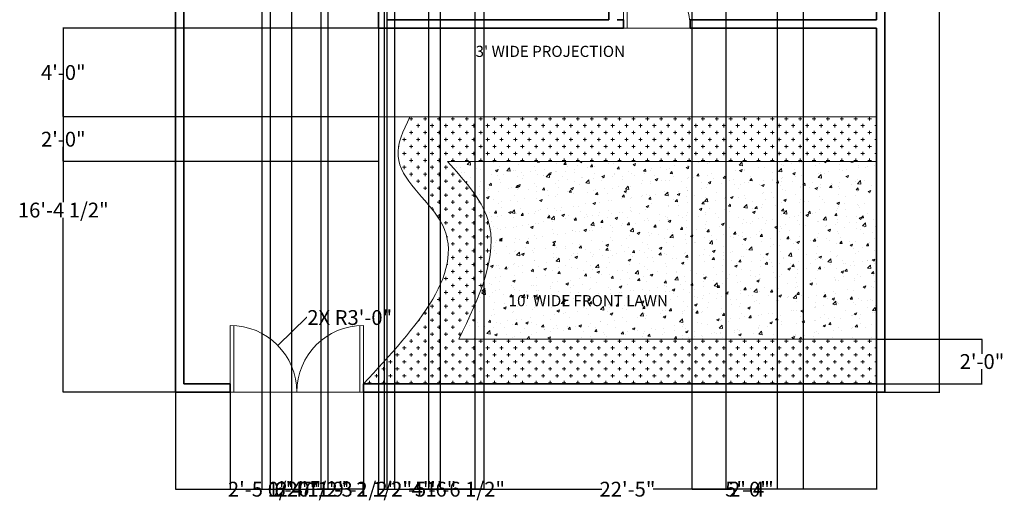
# Model space of a CAD drawing. Units: inches. Extents: x -438 to 102, y -60 to 1091.
# Tile 1 of 20: x -438 to 93, y -60 to 205. Entities that reach past the tile are written whole.
import ezdxf

# ---------------------------------------------------------------- set-up
doc = ezdxf.new("R2010")
doc.units = ezdxf.units.IN
doc.header["$MEASUREMENT"] = 0
for name, color, linetype, lineweight, true_color in [('A-ANNO-DIMS', 217, 'Continuous', 18, 0x93278f), ('A-DOOR', 30, 'Continuous', 18, 0xf26722), ('A-WALL', 2, 'Continuous', 35, 0xf1eb1f), ('C-PROP', 2, 'Continuous', 35, 0xf1eb1f), ('L-PLNT-PATT', 85, 'Continuous', 13, 0x58ba48)]:
    doc.layers.add(name, color=color, linetype=linetype, lineweight=lineweight, true_color=true_color)
for name, color, linetype, lineweight in [('A-AREA-IDEN', 4, 'Continuous', 18), ('C-SITE-GATE', 7, 'Continuous', 18), ('C-SITE-PVMT', 7, 'Continuous', 18), ('L-PLNT', 85, 'Continuous', 18)]:
    doc.layers.add(name, color=color, linetype=linetype, lineweight=lineweight)
doc.styles.get("Standard").update_dxf_attribs({"font": 'arial.ttf'})
doc.dimstyles.get("Standard").update_dxf_attribs({"dimtxt": 8, "dimasz": 0.18, "dimexe": 0.18, "dimexo": 0.0625, "dimgap": 0.09, "dimtad": 0, "dimtih": 1, "dimtoh": 1, "dimdec": 4, "dimzin": 0, "dimdsep": 46, "dimlunit": 3, "dimtxsty": 'Standard', "dimcen": 0.09, "dimadec": 0, "dimazin": 0, "dimtfac": 1, "dimtdec": 4, "dimtofl": 0, "dimtmove": 0, "dimatfit": 3, "dimfxl": 1, "dimtolj": 1, "dimtzin": 0, "dimarcsym": 0})

# ---------------------------------------------------------------- blocks, each defined once
blk = doc.blocks.new('*D5')
at = {"layer": 'A-ANNO-DIMS', "color": 0, "lineweight": -2, "transparency": 16777216}
for p, q in [((28.92, 1027), (58.42, 1027)), ((58.24, 1026.82), (58.24, 519.68)), ((58.24, 4.18), (58.24, 511.32)), ((28.92, 4), (58.42, 4))]:
    blk.add_line(p, q, dxfattribs=at)
at = {"layer": 'A-ANNO-DIMS', "color": 0, "transparency": 16777216}
for points in [[(58.21, 1026.82), (58.27, 1026.82), (58.24, 1027)], [(58.21, 4.18), (58.27, 4.18), (58.24, 4)]]:
    blk.add_solid(points, dxfattribs=at)
at = {"layer": 'Defpoints', "color": 0, "transparency": 16777216}
for p in [(28.85, 1027), (28.85, 4), (58.24, 4)]:
    blk.add_point(p, dxfattribs=at)
at = {"layer": 'A-ANNO-DIMS', "color": 0, "transparency": 16777216, "insert": (58.24, 515.5), "char_height": 8, "attachment_point": 5}
blk.add_mtext('\\A1;85\'-3.0000"', dxfattribs=at)
blk = doc.blocks.new('DOOR-SWING-36')
for p, q in [((-36, 0), (0, 0)), ((-2, 0), (-2, -36)), ((0, 0), (0, -36))]:
    blk.add_line(p, q)
blk.add_arc((0, 0), 36, 180, 270)
blk = doc.blocks.new('*D24')
at = {"layer": 'A-ANNO-DIMS', "color": 0, "lineweight": -2, "transparency": 16777216}
for p, q in [((-354.15, 3.94), (-354.15, -48.58)), ((-324.71, 3.94), (-324.71, -48.58)), ((-353.97, -48.4), (-324.89, -48.4)), ((-324.71, -48.4), (-324.53, -48.4))]:
    blk.add_line(p, q, dxfattribs=at)
at = {"layer": 'A-ANNO-DIMS', "color": 0, "transparency": 16777216}
for points in [[(-353.97, -48.37), (-353.97, -48.43), (-354.15, -48.4)], [(-324.89, -48.37), (-324.89, -48.43), (-324.71, -48.4)]]:
    blk.add_solid(points, dxfattribs=at)
at = {"layer": 'Defpoints', "color": 0, "transparency": 16777216}
for p in [(-354.15, 4), (-324.71, 4), (-324.71, -48.4)]:
    blk.add_point(p, dxfattribs=at)
at = {"layer": 'A-ANNO-DIMS', "color": 0, "transparency": 16777216, "insert": (-304.42, -48.4), "char_height": 8, "attachment_point": 5}
blk.add_mtext('\\A1;2\'-5 1/2"', dxfattribs=at)
blk = doc.blocks.new('*D25')
at = {"layer": 'A-ANNO-DIMS', "color": 0, "lineweight": -2, "transparency": 16777216}
for p, q in [((-324.71, 3.94), (-324.71, -48.58)), ((-252.71, 3.94), (-252.71, -48.58)), ((-324.53, -48.4), (-299.45, -48.4)), ((-252.89, -48.4), (-277.96, -48.4))]:
    blk.add_line(p, q, dxfattribs=at)
at = {"layer": 'A-ANNO-DIMS', "color": 0, "transparency": 16777216}
for points in [[(-324.53, -48.37), (-324.53, -48.43), (-324.71, -48.4)], [(-252.89, -48.37), (-252.89, -48.43), (-252.71, -48.4)]]:
    blk.add_solid(points, dxfattribs=at)
at = {"layer": 'Defpoints', "color": 0, "transparency": 16777216}
for p in [(-324.71, 4), (-252.71, 4), (-252.71, -48.4)]:
    blk.add_point(p, dxfattribs=at)
at = {"layer": 'A-ANNO-DIMS', "color": 0, "transparency": 16777216, "insert": (-288.71, -48.4), "char_height": 8, "attachment_point": 5}
blk.add_mtext('\\A1;6\'-0"', dxfattribs=at)
blk = doc.blocks.new('*D26')
at = {"layer": 'A-ANNO-DIMS', "color": 0, "lineweight": -2, "transparency": 16777216}
for p, q in [((-244.65, 200.44), (-244.65, -48.58)), ((24.35, 200.44), (24.35, -48.58)), ((-244.47, -48.4), (-124.05, -48.4)), ((24.17, -48.4), (-96.25, -48.4))]:
    blk.add_line(p, q, dxfattribs=at)
at = {"layer": 'A-ANNO-DIMS', "color": 0, "transparency": 16777216}
for points in [[(-244.47, -48.37), (-244.47, -48.43), (-244.65, -48.4)], [(24.17, -48.37), (24.17, -48.43), (24.35, -48.4)]]:
    blk.add_solid(points, dxfattribs=at)
at = {"layer": 'Defpoints', "color": 0, "transparency": 16777216}
for p in [(-244.65, 200.5), (24.35, 200.5), (24.35, -48.4)]:
    blk.add_point(p, dxfattribs=at)
at = {"layer": 'A-ANNO-DIMS', "color": 0, "transparency": 16777216, "insert": (-110.15, -48.4), "char_height": 8, "attachment_point": 5}
blk.add_mtext('\\A1;22\'-5"', dxfattribs=at)
blk = doc.blocks.new('*D27')
at = {"layer": 'A-ANNO-DIMS', "color": 0, "lineweight": -2, "transparency": 16777216}
for p, q in [((-244.71, 200.5), (-414.94, 200.5)), ((-414.76, 200.32), (-414.76, 106.48)), ((-414.76, 4.18), (-414.76, 98.02)), ((-354.21, 4), (-414.94, 4))]:
    blk.add_line(p, q, dxfattribs=at)
at = {"layer": 'A-ANNO-DIMS', "color": 0, "transparency": 16777216}
for points in [[(-414.79, 200.32), (-414.73, 200.32), (-414.76, 200.5)], [(-414.79, 4.18), (-414.73, 4.18), (-414.76, 4)]]:
    blk.add_solid(points, dxfattribs=at)
at = {"layer": 'Defpoints', "color": 0, "transparency": 16777216}
for p in [(-414.76, 200.5), (-244.65, 200.5), (-354.15, 4)]:
    blk.add_point(p, dxfattribs=at)
at = {"layer": 'A-ANNO-DIMS', "color": 0, "transparency": 16777216, "insert": (-414.76, 102.25), "char_height": 8, "attachment_point": 5}
blk.add_mtext('\\A1;16\'-4 1/2"', dxfattribs=at)
blk = doc.blocks.new('*D28')
at = {"layer": 'A-ANNO-DIMS', "color": 0, "lineweight": -2, "transparency": 16777216}
for p, q in [((-303.15, 353.94), (-303.15, -48.58)), ((-271.99, 353.94), (-271.99, -48.58)), ((-302.97, -48.4), (-298.36, -48.4)), ((-272.17, -48.4), (-276.78, -48.4))]:
    blk.add_line(p, q, dxfattribs=at)
at = {"layer": 'A-ANNO-DIMS', "color": 0, "transparency": 16777216}
for points in [[(-302.97, -48.37), (-302.97, -48.43), (-303.15, -48.4)], [(-272.17, -48.37), (-272.17, -48.43), (-271.99, -48.4)]]:
    blk.add_solid(points, dxfattribs=at)
at = {"layer": 'Defpoints', "color": 0, "transparency": 16777216}
for p in [(-303.15, 354), (-271.99, 354), (-271.99, -48.4)]:
    blk.add_point(p, dxfattribs=at)
at = {"layer": 'A-ANNO-DIMS', "color": 0, "transparency": 16777216, "insert": (-287.57, -48.4), "char_height": 8, "attachment_point": 5}
blk.add_mtext('\\A1;2\'-7"', dxfattribs=at)
blk = doc.blocks.new('*D29')
at = {"layer": 'A-ANNO-DIMS', "color": 0, "lineweight": -2, "transparency": 16777216}
for p, q in [((-303.15, 494.44), (-303.15, -48.58)), ((-192.65, 494.44), (-192.65, -48.58)), ((-302.97, -48.4), (-267.94, -48.4)), ((-192.83, -48.4), (-227.85, -48.4))]:
    blk.add_line(p, q, dxfattribs=at)
at = {"layer": 'A-ANNO-DIMS', "color": 0, "transparency": 16777216}
for points in [[(-302.97, -48.37), (-302.97, -48.43), (-303.15, -48.4)], [(-192.83, -48.37), (-192.83, -48.43), (-192.65, -48.4)]]:
    blk.add_solid(points, dxfattribs=at)
at = {"layer": 'Defpoints', "color": 0, "transparency": 16777216}
for p in [(-303.15, 494.5), (-192.65, 494.5), (-192.65, -48.4)]:
    blk.add_point(p, dxfattribs=at)
at = {"layer": 'A-ANNO-DIMS', "color": 0, "transparency": 16777216, "insert": (-247.9, -48.4), "char_height": 8, "attachment_point": 5}
blk.add_mtext('\\A1;9\'-2 1/2"', dxfattribs=at)
blk = doc.blocks.new('*D31')
at = {"layer": 'A-ANNO-DIMS', "color": 0, "lineweight": -2, "transparency": 16777216}
for p, q in [((-75.33, 454.94), (-75.33, -48.58)), ((-15.33, 454.94), (-15.33, -48.58)), ((-75.15, -48.4), (-56.05, -48.4)), ((-15.51, -48.4), (-34.6, -48.4))]:
    blk.add_line(p, q, dxfattribs=at)
at = {"layer": 'A-ANNO-DIMS', "color": 0, "transparency": 16777216}
for points in [[(-75.15, -48.37), (-75.15, -48.43), (-75.33, -48.4)], [(-15.51, -48.37), (-15.51, -48.43), (-15.33, -48.4)]]:
    blk.add_solid(points, dxfattribs=at)
at = {"layer": 'Defpoints', "color": 0, "transparency": 16777216}
for p in [(-75.33, 455), (-15.33, 455), (-15.33, -48.4)]:
    blk.add_point(p, dxfattribs=at)
at = {"layer": 'A-ANNO-DIMS', "color": 0, "transparency": 16777216, "insert": (-45.33, -48.4), "char_height": 8, "attachment_point": 5}
blk.add_mtext('\\A1;5\'-0"', dxfattribs=at)
blk = doc.blocks.new('*D32')
at = {"layer": 'A-ANNO-DIMS', "color": 0, "lineweight": -2, "transparency": 16777216}
for p, q in [((-307.65, 579.94), (-307.65, -48.58)), ((-303.15, 584.44), (-303.15, -48.58)), ((-307.47, -48.4), (-303.33, -48.4)), ((-303.15, -48.4), (-302.97, -48.4))]:
    blk.add_line(p, q, dxfattribs=at)
at = {"layer": 'A-ANNO-DIMS', "color": 0, "transparency": 16777216}
for points in [[(-307.47, -48.37), (-307.47, -48.43), (-307.65, -48.4)], [(-303.33, -48.37), (-303.33, -48.43), (-303.15, -48.4)]]:
    blk.add_solid(points, dxfattribs=at)
at = {"layer": 'Defpoints', "color": 0, "transparency": 16777216}
for p in [(-307.65, 580), (-303.15, 584.5), (-303.15, -48.4)]:
    blk.add_point(p, dxfattribs=at)
at = {"layer": 'A-ANNO-DIMS', "color": 0, "transparency": 16777216, "insert": (-282.92, -48.4), "char_height": 8, "attachment_point": 5}
blk.add_mtext('\\A1;0\'-4 1/2"', dxfattribs=at)
blk = doc.blocks.new('*D33')
at = {"layer": 'A-ANNO-DIMS', "color": 0, "lineweight": -2, "transparency": 16777216}
for p, q in [((-240.15, 349.44), (-240.15, -48.58)), ((-211.32, 349.44), (-211.32, -48.58)), ((-239.97, -48.4), (-236.52, -48.4)), ((-211.5, -48.4), (-214.94, -48.4))]:
    blk.add_line(p, q, dxfattribs=at)
at = {"layer": 'A-ANNO-DIMS', "color": 0, "transparency": 16777216}
for points in [[(-239.97, -48.37), (-239.97, -48.43), (-240.15, -48.4)], [(-211.5, -48.37), (-211.5, -48.43), (-211.32, -48.4)]]:
    blk.add_solid(points, dxfattribs=at)
at = {"layer": 'Defpoints', "color": 0, "transparency": 16777216}
for p in [(-240.15, 349.5), (-211.32, 349.5), (-211.32, -48.4)]:
    blk.add_point(p, dxfattribs=at)
at = {"layer": 'A-ANNO-DIMS', "color": 0, "transparency": 16777216, "insert": (-225.73, -48.4), "char_height": 8, "attachment_point": 5}
blk.add_mtext('\\A1;2\'-5"', dxfattribs=at)
blk = doc.blocks.new('*D35')
at = {"layer": 'A-ANNO-DIMS', "color": 0, "lineweight": -2, "transparency": 16777216}
for p, q in [((-57.12, 262.42), (-57.12, -48.58)), ((-29.37, 262.42), (-29.37, -48.58)), ((-56.94, -48.4), (-54.03, -48.4)), ((-29.55, -48.4), (-32.45, -48.4))]:
    blk.add_line(p, q, dxfattribs=at)
at = {"layer": 'A-ANNO-DIMS', "color": 0, "transparency": 16777216}
for points in [[(-56.94, -48.37), (-56.94, -48.43), (-57.12, -48.4)], [(-29.55, -48.37), (-29.55, -48.43), (-29.37, -48.4)]]:
    blk.add_solid(points, dxfattribs=at)
at = {"layer": 'Defpoints', "color": 0, "transparency": 16777216}
for p in [(-57.12, 262.49), (-29.37, 262.49), (-29.37, -48.4)]:
    blk.add_point(p, dxfattribs=at)
at = {"layer": 'A-ANNO-DIMS', "color": 0, "transparency": 16777216, "insert": (-43.24, -48.4), "char_height": 8, "attachment_point": 5}
blk.add_mtext('\\A1;2\'-4"', dxfattribs=at)
blk = doc.blocks.new('*D40')
at = {"layer": 'A-ANNO-DIMS', "color": 0, "lineweight": -2, "transparency": 16777216}
for p, q in [((-235.98, 270.35), (-235.98, -48.58)), ((-217.6, 270.35), (-217.6, -48.58)), ((-235.8, -48.4), (-217.78, -48.4)), ((-217.6, -48.4), (-217.42, -48.4))]:
    blk.add_line(p, q, dxfattribs=at)
at = {"layer": 'A-ANNO-DIMS', "color": 0, "transparency": 16777216}
for points in [[(-235.8, -48.37), (-235.8, -48.43), (-235.98, -48.4)], [(-217.78, -48.37), (-217.78, -48.43), (-217.6, -48.4)]]:
    blk.add_solid(points, dxfattribs=at)
at = {"layer": 'Defpoints', "color": 0, "transparency": 16777216}
for p in [(-235.98, 270.42), (-217.6, 270.42), (-217.6, -48.4)]:
    blk.add_point(p, dxfattribs=at)
at = {"layer": 'A-ANNO-DIMS', "color": 0, "transparency": 16777216, "insert": (-197.75, -48.4), "char_height": 8, "attachment_point": 5}
blk.add_mtext('\\A1;1\'-6 1/2"', dxfattribs=at)
blk = doc.blocks.new('*D51')
at = {"layer": 'A-ANNO-DIMS', "color": 0, "lineweight": -2, "transparency": 16777216}
for p, q in [((-291.54, 847), (-291.54, -48.58)), ((-275.79, 847), (-275.79, -48.58)), ((-291.36, -48.4), (-275.97, -48.4)), ((-275.79, -48.4), (-275.61, -48.4))]:
    blk.add_line(p, q, dxfattribs=at)
at = {"layer": 'A-ANNO-DIMS', "color": 0, "transparency": 16777216}
for points in [[(-291.36, -48.37), (-291.36, -48.43), (-291.54, -48.4)], [(-275.97, -48.37), (-275.97, -48.43), (-275.79, -48.4)]]:
    blk.add_solid(points, dxfattribs=at)
at = {"layer": 'Defpoints', "color": 0, "transparency": 16777216}
for p in [(-291.54, 847.06), (-275.79, 847.06), (-275.79, -48.4)]:
    blk.add_point(p, dxfattribs=at)
at = {"layer": 'A-ANNO-DIMS', "color": 0, "transparency": 16777216, "insert": (-255.95, -48.4), "char_height": 8, "attachment_point": 5}
blk.add_mtext('\\A1;1\'-3 1/2"', dxfattribs=at)
blk = doc.blocks.new('*D55')
at = {"layer": 'A-ANNO-DIMS', "color": 0, "lineweight": -2, "transparency": 16777216}
for p, q in [((-241.57, 808.32), (-241.57, -48.58)), ((-187.65, 801.94), (-187.65, -48.58)), ((-241.39, -48.4), (-225.49, -48.4)), ((-187.83, -48.4), (-203.72, -48.4))]:
    blk.add_line(p, q, dxfattribs=at)
at = {"layer": 'A-ANNO-DIMS', "color": 0, "transparency": 16777216}
for points in [[(-241.39, -48.37), (-241.39, -48.43), (-241.57, -48.4)], [(-187.83, -48.37), (-187.83, -48.43), (-187.65, -48.4)]]:
    blk.add_solid(points, dxfattribs=at)
at = {"layer": 'Defpoints', "color": 0, "transparency": 16777216}
for p in [(-241.57, 808.38), (-187.65, 802), (-187.65, -48.4)]:
    blk.add_point(p, dxfattribs=at)
at = {"layer": 'A-ANNO-DIMS', "color": 0, "transparency": 16777216, "insert": (-214.61, -48.4), "char_height": 8, "attachment_point": 5}
blk.add_mtext('\\A1;4\'-6"', dxfattribs=at)
blk = doc.blocks.new('*D57')
at = {"layer": 'A-ANNO-DIMS', "color": 0, "lineweight": -2, "transparency": 16777216}
for p, q in [((-244.71, 200.5), (-414.94, 200.5)), ((-414.76, 200.32), (-414.76, 180.67)), ((-414.76, 152.68), (-414.76, 172.32)), ((-244.71, 152.5), (-414.94, 152.5))]:
    blk.add_line(p, q, dxfattribs=at)
at = {"layer": 'A-ANNO-DIMS', "color": 0, "transparency": 16777216}
for points in [[(-414.79, 200.32), (-414.73, 200.32), (-414.76, 200.5)], [(-414.79, 152.68), (-414.73, 152.68), (-414.76, 152.5)]]:
    blk.add_solid(points, dxfattribs=at)
at = {"layer": 'Defpoints', "color": 0, "transparency": 16777216}
for p in [(-414.76, 200.5), (-244.65, 200.5), (-244.65, 152.5)]:
    blk.add_point(p, dxfattribs=at)
at = {"layer": 'A-ANNO-DIMS', "color": 0, "transparency": 16777216, "insert": (-414.76, 176.5), "char_height": 8, "attachment_point": 5}
blk.add_mtext('\\A1;4\'-0"', dxfattribs=at)
blk = doc.blocks.new('*D58')
at = {"layer": 'A-ANNO-DIMS', "color": 0, "lineweight": -2, "transparency": 16777216}
for p, q in [((-244.71, 152.5), (-414.94, 152.5)), ((-414.76, 152.32), (-414.76, 144.67)), ((-414.76, 128.68), (-414.76, 136.32)), ((-244.71, 128.5), (-414.94, 128.5))]:
    blk.add_line(p, q, dxfattribs=at)
at = {"layer": 'A-ANNO-DIMS', "color": 0, "transparency": 16777216}
for points in [[(-414.79, 152.32), (-414.73, 152.32), (-414.76, 152.5)], [(-414.79, 128.68), (-414.73, 128.68), (-414.76, 128.5)]]:
    blk.add_solid(points, dxfattribs=at)
at = {"layer": 'Defpoints', "color": 0, "transparency": 16777216}
for p in [(-414.76, 152.5), (-244.65, 152.5), (-244.65, 128.5)]:
    blk.add_point(p, dxfattribs=at)
at = {"layer": 'A-ANNO-DIMS', "color": 0, "transparency": 16777216, "insert": (-414.76, 140.5), "char_height": 8, "attachment_point": 5}
blk.add_mtext('\\A1;2\'-0"', dxfattribs=at)
blk = doc.blocks.new('*D59')
at = {"layer": 'A-ANNO-DIMS', "color": 0, "lineweight": -2, "transparency": 16777216}
for p, q in [((24.42, 32.5), (81.43, 32.5)), ((81.25, 32.32), (81.25, 24.67)), ((81.25, 8.68), (81.25, 16.32)), ((24.42, 8.5), (81.43, 8.5))]:
    blk.add_line(p, q, dxfattribs=at)
at = {"layer": 'A-ANNO-DIMS', "color": 0, "transparency": 16777216}
for points in [[(81.22, 32.32), (81.28, 32.32), (81.25, 32.5)], [(81.22, 8.68), (81.28, 8.68), (81.25, 8.5)]]:
    blk.add_solid(points, dxfattribs=at)
at = {"layer": 'Defpoints', "color": 0, "transparency": 16777216}
for p in [(24.35, 32.5), (81.25, 32.5), (24.35, 8.5)]:
    blk.add_point(p, dxfattribs=at)
at = {"layer": 'A-ANNO-DIMS', "color": 0, "transparency": 16777216, "insert": (81.25, 20.5), "char_height": 8, "attachment_point": 5}
blk.add_mtext('\\A1;2\'-0"', dxfattribs=at)
blk = doc.blocks.new('*D65')
at = {"layer": 'A-ANNO-DIMS', "color": 0, "lineweight": -2, "transparency": 16777216}
for p, q in [((-283.5, 44.25), (-298.83, 29.28)), ((-283.32, 44.25), (-283.5, 44.25)), ((-324.8, 4), (-324.62, 4)), ((-324.71, 3.91), (-324.71, 4.09))]:
    blk.add_line(p, q, dxfattribs=at)
at = {"layer": 'A-ANNO-DIMS', "color": 0, "transparency": 16777216}
blk.add_solid([(-298.85, 29.3), (-298.8, 29.26), (-298.95, 29.15)], dxfattribs=at)
at = {"layer": 'Defpoints', "color": 0, "transparency": 16777216}
for p in [(-298.95, 29.15), (-324.71, 4)]:
    blk.add_point(p, dxfattribs=at)
at = {"layer": 'A-ANNO-DIMS', "color": 0, "transparency": 16777216, "insert": (-260.11, 44.25), "char_height": 8, "attachment_point": 5}
blk.add_mtext('\\A1;2X R3\'-0"', dxfattribs=at)

msp = doc.modelspace()

# ---------------------------------------------------------------- hatches: boundary and pattern name
at = {"layer": 'L-PLNT-PATT'}
h = msp.add_hatch(dxfattribs=at)
h.set_pattern_fill('CROSS', color=256, scale=15)
h.set_pattern_definition([(0, (-842.8506, -448.43), (3.75, 3.75), [1.875, -5.625]), (90, (-841.913, -449.3675), (-3.75, 3.75), [1.875, -5.625])])
edge = h.paths.add_edge_path()
edge.add_line((24.35351, 152.49939), (-227.70947, 152.49939))
edge.add_spline(control_points=[(-227.70947, 152.49939), (-231.13031, 145.25083), (-240.91412, 124.51956), (-183.32461, 83.0062), (-224.06068, 39.26154), (-252.70713, 8.49939)], knot_values=[0, 0, 0, 0, 22.123250708, 63.273633799, 160.779688201, 160.779688201, 160.779688201, 160.779688201], degree=3, periodic=0)
edge.add_line((-252.70713, 8.49939), (24.35351, 8.49939))
edge.add_line((24.35351, 8.49939), (24.35351, 32.49939))
edge.add_line((24.35351, 32.49939), (-201.20088, 32.49939))
edge.add_spline(control_points=[(-201.20088, 32.49939), (-190.29613, 55.13304), (-173.13689, 90.7484), (-198.24399, 118.41499), (-207.39546, 128.49939)], knot_values=[0, 0, 0, 0, 66.555541517, 104.728967017, 104.728967017, 104.728967017, 104.728967017], degree=3, periodic=0)
edge.add_line((-207.39546, 128.49939), (24.35351, 128.49939))
edge.add_line((24.35351, 128.49939), (24.35351, 152.49939))
h = msp.add_hatch(dxfattribs=at)
h.set_pattern_fill('AR-CONC', color=256, scale=2)
h.set_pattern_definition([(50, (-842.851, -448.43), (14.3452, -1.25504), [1.5, -16.5]), (355, (-842.85, -448.43), (-2.77503, 15.04384), [1.2, -13.2]), (100.4514, (-841.655, -448.535), (11.57018, 13.7888), [1.2748, -14.02284]), (46.1842, (-842.85, -444.43), (21.34483, -3.3104), [2.25, -24.75]), (96.6356, (-841.072, -444.706), (18.69324, 19.48237), [1.9122, -21.03428]), (351.1842, (-842.85, -444.43), (18.69324, 19.48237), [1.8, -19.8]), (21, (-840.851, -445.43), (11.93814, -8.05238), [1.5, -16.5]), (326, (-840.85, -445.43), (4.8663, 14.503), [1.2, -13.2]), (71.4514, (-839.856, -446.101), (16.80445, 6.45062), [1.2748, -14.02284]), (37.5, (-842.8506, -448.43), (0.243197, 6.657877), [0, -13.04, 0, -13.4, 0, -13.25]), (7.5, (-842.8506, -448.43), (5.26139, 7.888234), [0, -7.64, 0, -12.74, 0, -5.05]), (327.5, (-847.3106, -448.43), (10.67645, -0.451097), [0, -5, 0, -15.6, 0, -20.7]), (317.5, (-849.311, -448.43), (11.66372, 2.0021), [0, -6.5, 0, -10.36, 0, -14.7])])
edge = h.paths.add_edge_path()
edge.add_line((24.35351, 128.49939), (-207.39546, 128.49939))
edge.add_spline(control_points=[(-207.39546, 128.49939), (-198.24399, 118.41499), (-173.13689, 90.7484), (-190.29613, 55.13304), (-201.20088, 32.49939)], knot_values=[0, 0, 0, 0, 38.1734255, 104.728967017, 104.728967017, 104.728967017, 104.728967017], degree=3, periodic=0)
edge.add_line((-201.20088, 32.49939), (24.35351, 32.49939))
edge.add_line((24.35351, 32.49939), (24.35351, 128.49939))
h.paths.add_polyline_path([(-175.87321, 48.69578), (-79.89163, 48.69578), (-79.89163, 58.00888), (-175.87321, 58.00888)], flags=24)

# ---------------------------------------------------------------- linework, layer by layer
at = {"layer": 'A-WALL'}
for p, q in [((24.35351, 204.99939), (24.35351, 450.49939)), ((-244.64649, 200.49939), (-244.64649, 349.49939)), ((-120.14649, 204.99939), (-120.14649, 349.49939)), ((-120.14649, 204.99939), (-240.14649, 204.99939)), ((-112.33294, 204.99939), (-115.64649, 204.99939)), ((-112.33294, 204.99939), (-112.33294, 200.49939)), ((24.35351, 204.99939), (-76.33294, 204.99939)), ((-76.33294, 204.99939), (-76.33294, 200.49939)), ((-112.33294, 200.49939), (-244.64649, 200.49939)), ((24.35351, 200.49939), (-76.33294, 200.49939))]:
    msp.add_line(p, q, dxfattribs=at)
at = {"layer": 'C-PROP'}
for p, q in [((-354.14649, 1026.99939), (-354.14649, 3.99939)), ((28.85351, 3.99939), (28.85351, 1026.99939)), ((-349.64649, 897.99939), (-349.64649, 8.49939)), ((24.35351, 160.46045), (24.35351, 200.49939)), ((24.35351, 8.49939), (24.35351, 164.49939)), ((-324.70713, 8.49939), (-349.64649, 8.49939)), ((-324.70713, 8.49939), (-324.70713, 3.99939)), ((24.35351, 8.49939), (-252.70713, 8.49939)), ((-252.70713, 8.49939), (-252.70713, 3.99939)), ((-324.70713, 3.99939), (-354.14649, 3.99939)), ((28.85351, 3.99939), (-252.70713, 3.99939))]:
    msp.add_line(p, q, dxfattribs=at)
at = {"layer": 'C-SITE-GATE'}
for p, q in [((-324.70713, 3.99939), (-324.70713, 39.99939)), ((-322.70713, 3.99939), (-322.70713, 39.99939)), ((-254.70713, 3.99939), (-254.70713, 39.99939)), ((-252.70713, 3.99939), (-252.70713, 39.99939)), ((-324.70713, 3.99939), (-252.70713, 3.99939))]:
    msp.add_line(p, q, dxfattribs=at)
for centre, start, end in [((-324.70713, 3.99939), 0, 90), ((-252.70713, 3.99939), 90, 180)]:
    msp.add_arc(centre, 36, start, end, dxfattribs=at)
at = {"layer": 'C-SITE-PVMT'}
for p, q in [((-234.26022, 152.49939), (-244.64649, 152.49939)), ((-244.64649, 152.49939), (-244.64649, 128.49939)), ((-244.64649, 128.49939), (-349.64649, 128.49939))]:
    msp.add_line(p, q, dxfattribs=at)
at = {"layer": 'L-PLNT'}
for p, q in [((-234.26022, 152.49939), (24.35351, 152.49939)), ((-207.39546, 128.49939), (24.35351, 128.49939)), ((24.35351, 32.49939), (-201.20088, 32.49939))]:
    msp.add_line(p, q, dxfattribs=at)
for points, knots in [([(-227.70947, 152.49939), (-231.13031, 145.25083), (-240.91412, 124.51956), (-183.32461, 83.0062), (-224.06068, 39.26154), (-252.70713, 8.49939)], [0, 0, 0, 0, 22.123250708, 63.273633799, 160.779688201, 160.779688201, 160.779688201, 160.779688201]), ([(-207.39546, 128.49939), (-198.24399, 118.41499), (-173.13689, 90.7484), (-190.29613, 55.13304), (-201.20088, 32.49939)], [0, 0, 0, 0, 38.1734255, 104.728967017, 104.728967017, 104.728967017, 104.728967017])]:
    msp.add_open_spline(points, degree=3, knots=knots, dxfattribs=at)

# ---------------------------------------------------------------- block references
at = {"layer": 'A-DOOR', "rotation": 180}
msp.add_blockref('DOOR-SWING-36', (-112.33294, 200.49939), dxfattribs=at)

# ---------------------------------------------------------------- texts
at = {"layer": 'A-AREA-IDEN'}
for s, p in [("3' WIDE PROJECTION", (-192.15365, 184.90021)), ("10' WIDE FRONT LAWN", (-174.32103, 50.35028))]:
    msp.add_text(s, height=6, dxfattribs=at).set_placement(p)

# ---------------------------------------------------------------- dimensions: what is measured, and where the dimension line sits
at = {"layer": 'A-ANNO-DIMS'}
for base, p1, p2, override, picture, middle in [((58.24207, 3.99939), (28.85351, 1026.99939), (28.85351, 3.99939), {"dimclrd": 0, "dimclre": 0, "dimclrt": 0}, '*D5', (58.24207, 515.49939)), ((-414.76009, 200.49939), (-354.14649, 3.99939), (-244.64649, 200.49939), {"dimdec": 1, "dimlfac": 1, "dimrnd": 0, "dimzin": 1, "dimdsep": 46, "dimlunit": 4, "dimfrac": 2}, '*D27', (-414.76009, 102.24939)), ((-414.76009, 200.49939), (-244.64649, 152.49939), (-244.64649, 200.49939), {"dimdec": 1, "dimlfac": 1, "dimrnd": 0, "dimzin": 1, "dimdsep": 46, "dimlunit": 4, "dimfrac": 2}, '*D57', (-414.76009, 176.49939)), ((-414.76009, 152.49939), (-244.64649, 128.49939), (-244.64649, 152.49939), {"dimdec": 1, "dimlfac": 1, "dimrnd": 0, "dimzin": 1, "dimdsep": 46, "dimlunit": 4, "dimfrac": 2}, '*D58', (-414.76009, 140.49939)), ((81.25351, 32.49939), (24.35351, 8.49939), (24.35351, 32.49939), {"dimdec": 1, "dimlfac": 1, "dimrnd": 0, "dimzin": 1, "dimdsep": 46, "dimlunit": 4, "dimfrac": 2}, '*D59', (81.25351, 20.49939))]:
    dim = msp.add_linear_dim(base=base, p1=p1, p2=p2, angle=90, dimstyle='Standard', override=override, dxfattribs=at)
    dim.commit()
    dim.dimension.update_dxf_attribs({"geometry": picture, "text_midpoint": middle})
for base, p1, p2, picture, middle in [((-275.79225, -48.40061), (-291.54025, 847.06395), (-275.79225, 847.06395), '*D51', (-255.94517, -48.40061)), ((-187.64649, -48.40061), (-241.57044, 808.38394), (-187.64649, 801.99939), '*D55', (-214.60846, -48.40061)), ((-303.14649, -48.40061), (-307.64649, 579.99939), (-303.14649, 584.49939), '*D32', (-282.92287, -48.40061)), ((-192.64649, -48.40061), (-303.14649, 494.49939), (-192.64649, 494.49939), '*D29', (-247.89649, -48.40061)), ((-15.32797, -48.40061), (-75.32797, 454.99939), (-15.32797, 454.99939), '*D31', (-45.32797, -48.40061)), ((-271.98824, -48.40061), (-303.14649, 353.99939), (-271.98824, 353.99939), '*D28', (-287.56737, -48.40061)), ((-211.31973, -48.40061), (-240.14649, 349.49939), (-211.31973, 349.49939), '*D33', (-225.73311, -48.40061)), ((-217.59887, -48.40061), (-235.97515, 270.41548), (-217.59887, 270.41548), '*D40', (-197.75179, -48.40061)), ((-29.36624, -48.40061), (-57.12044, 262.4853), (-29.36624, 262.4853), '*D35', (-43.24334, -48.40061)), ((24.35351, -48.40061), (-244.64649, 200.49939), (24.35351, 200.49939), '*D26', (-110.14649, -48.40061)), ((-324.70713, -48.40061), (-354.14649, 3.99939), (-324.70713, 3.99939), '*D24', (-304.4153, -48.40061)), ((-252.70713, -48.40061), (-324.70713, 3.99939), (-252.70713, 3.99939), '*D25', (-288.70713, -48.40061))]:
    dim = msp.add_linear_dim(base=base, p1=p1, p2=p2, dimstyle='Standard', override={"dimdec": 1, "dimlfac": 1, "dimrnd": 0, "dimzin": 1, "dimdsep": 46, "dimlunit": 4, "dimfrac": 2}, dxfattribs=at)
    dim.commit()
    dim.dimension.update_dxf_attribs({"geometry": picture, "text_midpoint": middle})
dim = msp.add_radius_dim(center=(-324.70713, 3.99939), mpoint=(-298.95389, 29.15433), text='2X <>', dimstyle='Standard', override={"dimdec": 1, "dimlfac": 1, "dimrnd": 0, "dimzin": 1, "dimdsep": 46, "dimlunit": 4, "dimfrac": 2}, dxfattribs=at)
dim.commit()
dim.dimension.update_dxf_attribs({"geometry": '*D65', "text_midpoint": (-260.10781, 44.24729), "dimtype": 164})

doc.saveas('drawing.dxf')
